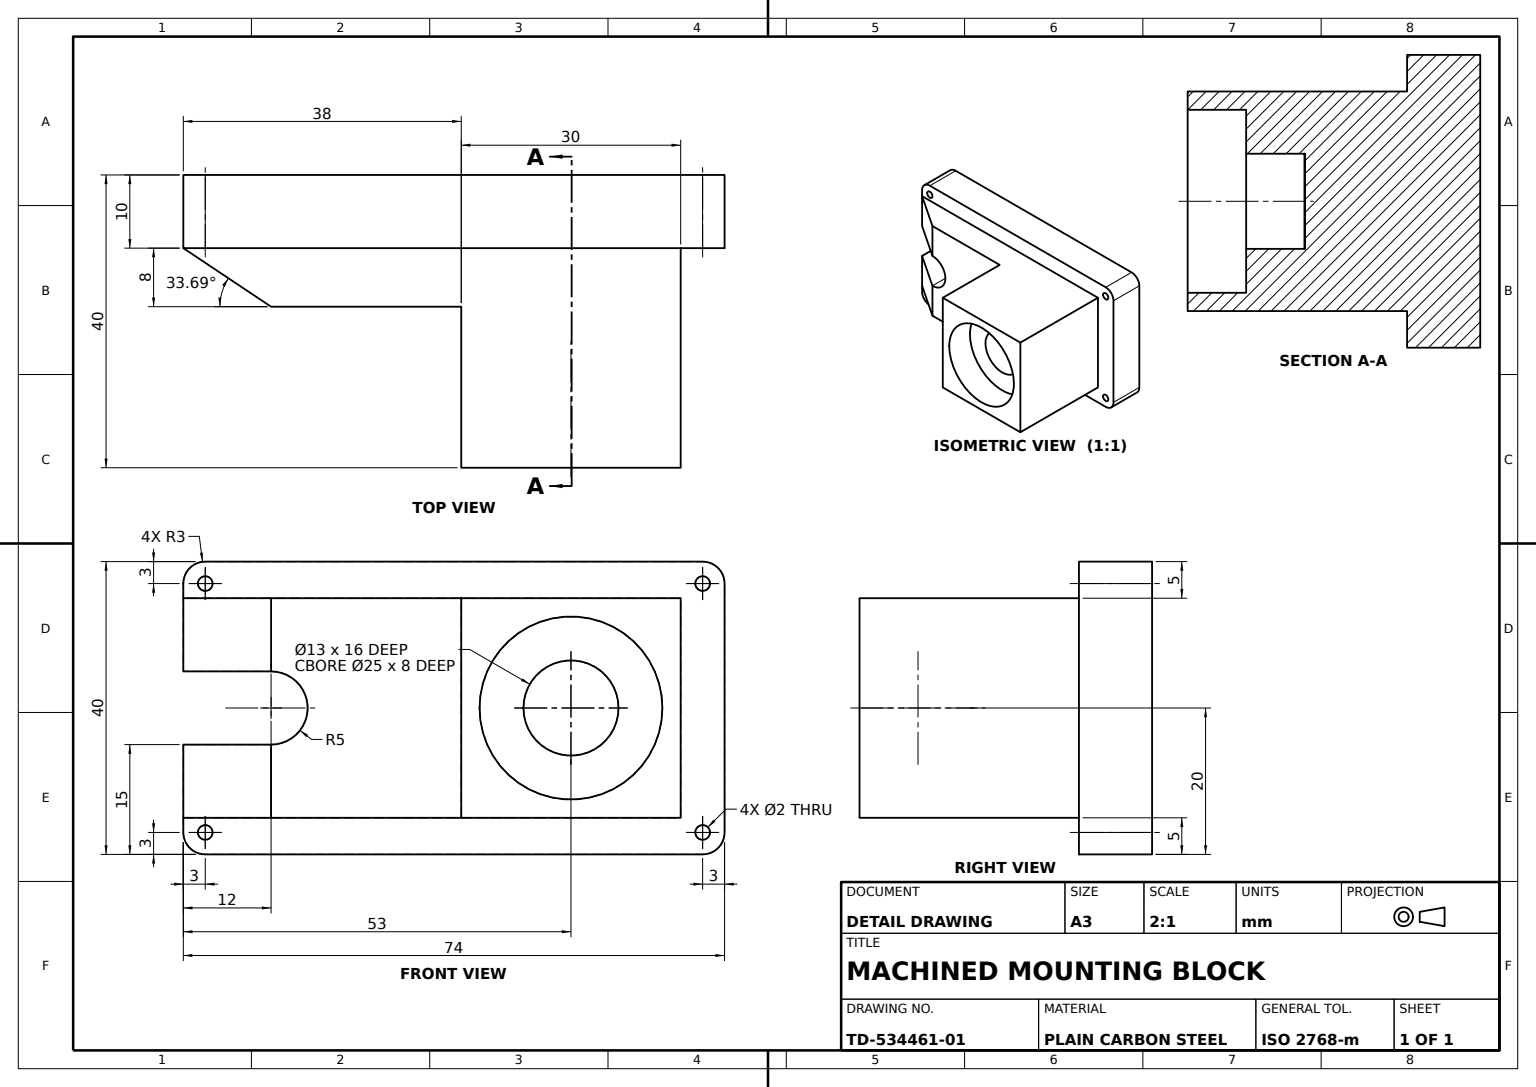
from build123d import *

# Parameters (mm, degrees)
MOUNTING_FLANGE_DEPTH    = 10
HOUSING_BLOCK_PROFILE_W  = 30
HOUSING_BLOCK_PROFILE_H  = 30
HOUSING_BLOCK_DEPTH      = 30
UPPER_BLOCK_PROFILE_W    = 8
UPPER_BLOCK_PROFILE_H    = 30
UPPER_BLOCK_DEPTH        = 26
SIDE_RELIEF_CUT_DEPTH    = 8
GUSSET_A_DEPTH           = 10
GUSSET_B_DEPTH           = 10
MOUNTING_HOLES_PROFILE_R = 1
MOUNTING_HOLES_4X_DEPTH  = 10
COUNTERBORE_25_PROFILE_R = 12.5
COUNTERBORE_25_DEPTH     = 8
BORE_13_PROFILE_R        = 6.5
BORE_13_DEPTH            = 8


with BuildPart() as part:
    # Flange Profile → Mounting Flange (new body)
    with BuildSketch(Plane.XY):
        with BuildLine():
            Line((3, 0), (71, 0))
            ThreePointArc((71, 0), (73.121320344, 0.878679656), (74, 3))
            Line((74, 3), (74, 37))
            ThreePointArc((74, 37), (73.121320344, 39.121320344), (71, 40))
            Line((71, 40), (3, 40))
            ThreePointArc((3, 40), (0.878679656, 39.121320344), (0, 37))
            Line((0, 37), (0, 25))
            Line((0, 25), (12, 25))
            ThreePointArc((12, 25), (17, 20), (12, 15))
            Line((12, 15), (0, 15))
            Line((0, 15), (0, 3))
            ThreePointArc((0, 3), (0.878679656, 0.878679656), (3, 0))
        make_face()
    extrude(amount=MOUNTING_FLANGE_DEPTH)

    # Housing Block Profile → Housing Block (add)
    with BuildSketch(Plane.XY.offset(10)):
        with Locations((53, 20)):
            Rectangle(HOUSING_BLOCK_PROFILE_W, HOUSING_BLOCK_PROFILE_H)
    extrude(amount=HOUSING_BLOCK_DEPTH)

    # Upper Block Profile → Upper Block (add)
    with BuildSketch(Plane.ZY.offset(-38)):
        with Locations((14, 20)):
            Rectangle(UPPER_BLOCK_PROFILE_W, UPPER_BLOCK_PROFILE_H)
    extrude(amount=UPPER_BLOCK_DEPTH)

    # Side Relief Profile → Side Relief Cut (cut)
    with BuildSketch(Plane(origin=(0, 0, 10), x_dir=(-1, 0, 0), z_dir=(0, 0, -1))):
        with BuildLine():
            Line((-12, 25), (-12, 15))
            ThreePointArc((-12, 15), (-17, 20), (-12, 25))
        make_face()
    extrude(amount=-SIDE_RELIEF_CUT_DEPTH, mode=Mode.SUBTRACT)

    # Gusset A Profile → Gusset A (add)
    with BuildSketch(Plane.XZ.offset(-5)):
        Polygon((12, 10), (12, 18), (0, 10), align=None)
    extrude(amount=-GUSSET_A_DEPTH)

    # Gusset B Profile → Gusset B (add)
    with BuildSketch(Plane(origin=(0, 35, 0), x_dir=(1, 0, 0), z_dir=(0, 1, 0))):
        Polygon((12, -18), (12, -10), (0, -10), align=None)
    extrude(amount=-GUSSET_B_DEPTH)

    # Mounting Holes Profile → Mounting Holes 4x (cut)
    with BuildSketch(Plane.XY.offset(10)):
        with Locations((3, 37)):
            Circle(MOUNTING_HOLES_PROFILE_R)
        with Locations((71, 37)):
            Circle(MOUNTING_HOLES_PROFILE_R)
        with Locations((71, 3)):
            Circle(MOUNTING_HOLES_PROFILE_R)
        with Locations((3, 3)):
            Circle(MOUNTING_HOLES_PROFILE_R)
    extrude(amount=-MOUNTING_HOLES_4X_DEPTH, mode=Mode.SUBTRACT)

    # Counterbore Ø25 Profile → Counterbore Ø25 (cut)
    with BuildSketch(Plane.XY.offset(40)):
        with Locations((53, 20)):
            Circle(COUNTERBORE_25_PROFILE_R)
    extrude(amount=-COUNTERBORE_25_DEPTH, mode=Mode.SUBTRACT)

    # Bore Ø13 Profile → Bore Ø13 (cut)
    with BuildSketch(Plane.XY.offset(32)):
        with Locations((53, 20)):
            Circle(BORE_13_PROFILE_R)
    extrude(amount=-BORE_13_DEPTH, mode=Mode.SUBTRACT)


solid = part.part
